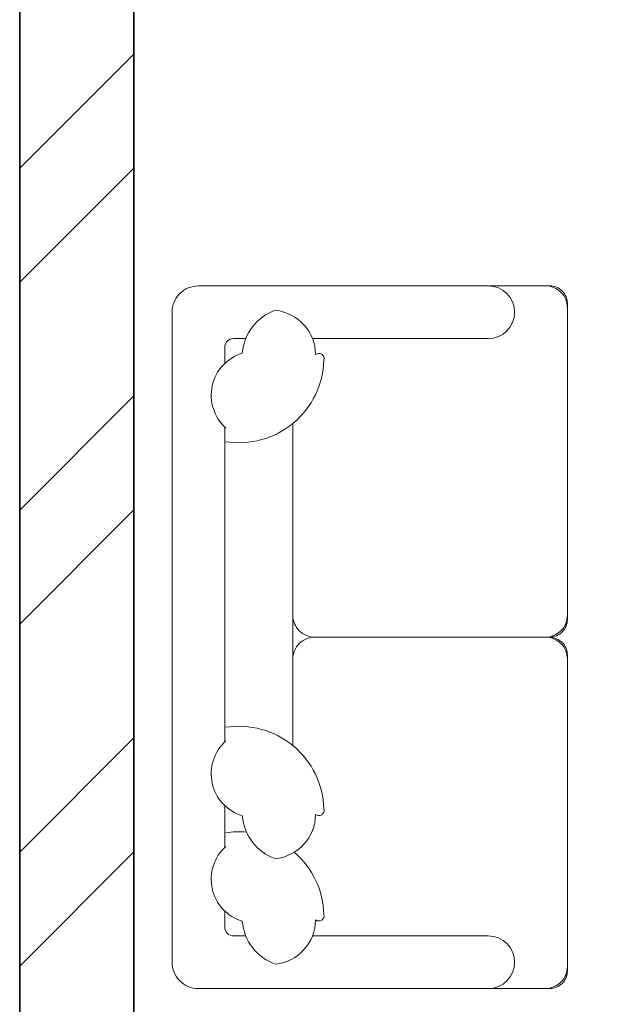
# Model space of a CAD drawing. Units: inches. Extents: x 2168 to 3056, y 1130 to 2629.
# Tile 10 of 42: x 2645 to 2669, y 1979 to 2018. Entities that reach past the tile are written whole.
import ezdxf

# ---------------------------------------------------------------- set-up
doc = ezdxf.new("R2010")
doc.units = ezdxf.units.IN
doc.layers.add('A-FURN', color=8, linetype='Continuous', lineweight=13)
doc.layers.add('A-WALL', color=7, linetype='Continuous', lineweight=35)
doc.layers.add('A-WALL-PATT', color=143, linetype='Continuous', lineweight=13, true_color=0x7aafdf)

msp = doc.modelspace()

# ---------------------------------------------------------------- hatches: boundary and pattern name
at = {"layer": 'A-WALL-PATT'}
h = msp.add_hatch(dxfattribs=at)
h.set_pattern_fill('ANSI32', color=256)
h.paths.add_polyline_path([(2463.796, 2409.389), (2467.387, 2409.389), (2467.387, 2413.889), (2454.768, 2413.889), (2454.768, 2411.639), (2454.768, 2409.389), (2459.296, 2409.389), (2459.296, 2265.389), (2455.644, 2265.389), (2455.644, 2260.889), (2467.349, 2260.889), (2467.349, 2263.139), (2467.349, 2265.389), (2463.796, 2265.389)])
h.paths.add_polyline_path([(2431.596, 2413.889), (2409.647, 2413.889), (2409.647, 2409.389), (2431.596, 2409.389), (2431.596, 2411.639)])
h.paths.add_polyline_path([(2349.647, 2413.889), (2331.796, 2413.889), (2331.796, 2362.671), (2336.296, 2362.671), (2336.296, 2409.389), (2349.647, 2409.389), (2349.647, 2411.639)])
h.paths.add_polyline_path([(2634.149, 2411.639), (2634.149, 2413.889), (2562.293, 2413.889), (2562.293, 2409.389), (2595.796, 2409.389), (2595.796, 2280.309), (2595.826, 2280.309), (2595.826, 2265.389), (2499.91, 2265.389), (2499.91, 2260.889), (2550.796, 2260.889), (2550.796, 2117.308), (2555.296, 2117.308), (2555.296, 2168.08), (2571.93, 2168.08), (2571.93, 2176.889), (2559.796, 2176.889), (2559.796, 2256.389), (2640.796, 2256.389), (2640.796, 2176.889), (2626.428, 2176.889), (2626.428, 2168.08), (2645.296, 2168.08), (2645.296, 2116.637), (2649.796, 2116.637), (2649.796, 2260.889), (2691.251, 2260.889), (2691.251, 2263.139), (2691.251, 2265.389), (2670.655, 2265.389), (2670.655, 2265.365), (2600.296, 2265.365), (2600.296, 2280.258), (2600.296, 2409.389), (2634.149, 2409.389)])
h.paths.add_polyline_path([(2600.296, 2473.889), (2612.84, 2473.889), (2612.84, 2478.389), (2572.636, 2478.389), (2572.636, 2473.889), (2595.796, 2473.889), (2595.796, 2413.889), (2600.296, 2413.889)])
h.paths.add_polyline_path([(2535.796, 2473.889), (2548.636, 2473.889), (2548.636, 2478.389), (2531.396, 2478.389), (2531.396, 2413.889), (2521.6, 2413.889), (2521.6, 2409.389), (2539.239, 2409.389), (2539.239, 2411.639), (2539.239, 2413.889), (2535.796, 2413.889)])
h.paths.add_polyline_path([(2664.796, 2478.389), (2636.84, 2478.389), (2636.84, 2473.889), (2660.296, 2473.889), (2660.296, 2413.889), (2656.165, 2413.889), (2656.165, 2409.389), (2671.684, 2409.389), (2671.684, 2411.639), (2671.684, 2413.889), (2664.796, 2413.889)])
h.paths.add_polyline_path([(2705.942, 2413.889), (2695.684, 2413.889), (2695.684, 2409.389), (2705.942, 2409.389)])
h.paths.add_polyline_path([(2741.35, 2413.889), (2728.733, 2413.889), (2728.733, 2411.639), (2728.733, 2409.389), (2732.296, 2409.389), (2732.296, 2265.389), (2725.733, 2265.389), (2725.733, 2260.889), (2740.917, 2260.889), (2740.917, 2263.139), (2740.917, 2265.389), (2736.796, 2265.389), (2736.796, 2409.389), (2741.35, 2409.389)])
h.paths.add_polyline_path([(2785.655, 2413.889), (2764.546, 2413.889), (2764.486, 2409.389), (2785.655, 2409.389), (2785.655, 2411.639)])
h.paths.add_polyline_path([(2864.296, 2413.889), (2845.655, 2413.889), (2845.655, 2409.389), (2859.796, 2409.389), (2859.796, 2368.425), (2864.296, 2368.425)])
h.paths.add_polyline_path([(2864.296, 2308.425), (2862.046, 2308.425), (2859.796, 2308.425), (2859.796, 2265.389), (2774.483, 2265.389), (2774.483, 2263.139), (2774.483, 2260.889), (2781.796, 2260.889), (2781.796, 2226.654), (2786.296, 2226.654), (2786.296, 2260.889), (2859.796, 2260.889), (2859.796, 2241.352), (2864.296, 2241.352)])
h.paths.add_polyline_path([(2864.296, 2217.352), (2862.046, 2217.352), (2859.796, 2217.352), (2859.796, 2200.889), (2786.296, 2200.889), (2786.296, 2205.931), (2784.046, 2205.931), (2781.796, 2205.931), (2781.796, 2150.974), (2786.296, 2150.974), (2786.296, 2161.889), (2859.796, 2161.889), (2859.796, 2144.419), (2864.296, 2144.419)])
h.paths.add_polyline_path([(2859.796, 2196.389), (2859.796, 2166.389), (2786.296, 2166.389), (2786.296, 2196.389)], flags=16)
h.paths.add_polyline_path([(2864.296, 2108.419), (2862.046, 2108.419), (2859.796, 2108.419), (2859.796, 2080.889), (2786.296, 2080.889), (2786.296, 2111.993), (2781.796, 2111.993), (2781.796, 2080.889), (2649.796, 2080.889), (2649.796, 2086.036), (2647.546, 2086.036), (2645.296, 2086.036), (2645.296, 2071.739), (2649.796, 2071.739), (2649.796, 2076.389), (2781.796, 2076.389), (2781.796, 2041.792), (2786.296, 2041.792), (2786.296, 2076.389), (2859.796, 2076.389), (2859.796, 2058.577), (2864.296, 2058.577)])
h.paths.add_polyline_path([(2864.296, 2022.577), (2859.796, 2022.577), (2859.796, 1992.389), (2786.296, 1992.389), (2786.296, 1999.573), (2781.796, 1999.573), (2781.796, 1848.085), (2784.046, 1848.085), (2786.296, 1848.085), (2786.296, 1851.389), (2859.796, 1851.389), (2859.796, 1838.258), (2864.296, 1838.258)], flags=17)
h.paths.add_polyline_path([(2859.796, 1987.889), (2859.796, 1855.889), (2786.296, 1855.889), (2786.296, 1987.889)], flags=16)
h.paths.add_polyline_path([(2823.046, 1987.889), (2841.421, 1921.889), (2823.046, 1855.889)], flags=0)
h.paths.add_polyline_path([(2864.296, 1814.258), (2859.796, 1814.258), (2859.796, 1791.389), (2786.296, 1791.389), (2786.296, 1825.658), (2784.046, 1825.658), (2781.796, 1825.658), (2781.796, 1791.389), (2720.155, 1791.389), (2720.155, 1791.265), (2649.796, 1791.265), (2649.796, 1806.159), (2649.796, 2038.983), (2647.546, 2038.983), (2645.296, 2038.983), (2645.296, 1783.925), (2649.796, 1783.925), (2649.796, 1786.889), (2781.796, 1786.889), (2781.796, 1746.789), (2786.296, 1746.789), (2786.296, 1786.889), (2859.796, 1786.889), (2859.796, 1770.083), (2864.296, 1770.083)])
h.paths.add_polyline_path([(2864.296, 1734.083), (2862.046, 1734.083), (2859.796, 1734.083), (2859.796, 1705.889), (2786.296, 1705.889), (2786.296, 1714.166), (2781.796, 1714.166), (2781.796, 1660.527), (2786.296, 1660.527), (2786.296, 1666.889), (2859.796, 1666.889), (2859.796, 1648.342), (2864.296, 1648.342)])
h.paths.add_polyline_path([(2786.296, 1701.389), (2859.796, 1701.389), (2859.796, 1671.389), (2786.296, 1671.389)], flags=16)
h.paths.add_polyline_path([(2649.796, 1756.576), (2647.546, 1756.576), (2645.296, 1756.576), (2645.296, 1606.889), (2555.296, 1606.889), (2555.296, 1749.513), (2553.046, 1749.513), (2550.796, 1749.513), (2550.796, 1606.889), (2503.006, 1606.889), (2503.006, 1604.639), (2503.006, 1602.389), (2595.796, 1602.389), (2595.849, 1602.389), (2595.849, 1587.495), (2595.796, 1458.389), (2561.502, 1458.389), (2561.502, 1456.139), (2561.502, 1453.889), (2595.796, 1453.889), (2595.796, 1381.889), (2573.438, 1381.889), (2573.438, 1377.389), (2613.01, 1377.389), (2613.01, 1379.639), (2613.01, 1381.889), (2600.296, 1381.889), (2600.296, 1453.889), (2634.327, 1453.889), (2634.327, 1458.389), (2600.296, 1458.389), (2600.296, 1602.389), (2670.655, 1602.389), (2694.095, 1602.389), (2694.095, 1606.889), (2649.796, 1606.889)])
h.paths.add_polyline_path([(2736.796, 1602.389), (2741.562, 1602.389), (2741.562, 1606.889), (2726.203, 1606.889), (2726.203, 1604.639), (2726.203, 1602.389), (2732.296, 1602.389), (2732.296, 1458.389), (2727.899, 1458.389), (2727.899, 1453.889), (2740.821, 1453.889), (2740.821, 1456.139), (2740.821, 1458.389), (2736.796, 1458.389)])
h.paths.add_polyline_path([(2859.796, 1606.889), (2786.296, 1606.889), (2786.296, 1637.334), (2784.046, 1637.334), (2781.796, 1637.334), (2781.796, 1606.889), (2775.612, 1606.889), (2775.612, 1602.389), (2859.796, 1602.389)])
h.paths.add_polyline_path([(2864.296, 1624.342), (2862.046, 1624.342), (2859.796, 1624.342), (2859.796, 1570.39), (2864.296, 1570.39)])
h.paths.add_polyline_path([(2864.296, 1510.39), (2862.046, 1510.39), (2859.796, 1510.39), (2859.796, 1458.389), (2846.735, 1458.389), (2846.735, 1456.139), (2846.735, 1453.889), (2864.296, 1453.889)])
h.paths.add_polyline_path([(2786.735, 1458.389), (2765.444, 1458.389), (2765.444, 1453.889), (2786.735, 1453.889)])
h.paths.add_polyline_path([(2706.004, 1458.389), (2695.36, 1458.389), (2695.36, 1453.889), (2706.004, 1453.889), (2706.004, 1456.139)])
h.paths.add_polyline_path([(2671.36, 1456.139), (2671.36, 1458.389), (2655.986, 1458.389), (2655.986, 1456.139), (2655.986, 1453.889), (2660.296, 1453.889), (2660.296, 1381.889), (2637.01, 1381.889), (2637.01, 1377.389), (2664.796, 1377.389), (2664.796, 1453.889), (2671.36, 1453.889)], flags=17)
h.paths.add_polyline_path([(2539.829, 1458.389), (2520.237, 1458.389), (2520.237, 1453.889), (2531.296, 1453.889), (2531.296, 1377.389), (2546.449, 1377.389), (2546.449, 1379.639), (2546.449, 1381.889), (2535.796, 1381.889), (2535.796, 1453.889), (2539.829, 1453.889)], flags=17)
h.paths.add_polyline_path([(2496.237, 1458.389), (2489.13, 1458.389), (2489.13, 1453.889), (2496.237, 1453.889), (2496.237, 1456.139)])
h.paths.add_polyline_path([(2467.433, 1456.139), (2467.433, 1458.389), (2463.796, 1458.389), (2463.796, 1602.389), (2468.242, 1602.389), (2468.242, 1605.7), (2468.242, 1606.889), (2454.602, 1606.889), (2454.602, 1602.389), (2459.296, 1602.389), (2459.296, 1458.389), (2454.24, 1458.389), (2454.24, 1453.889), (2467.433, 1453.889)])
h.paths.add_polyline_path([(2431.601, 1456.139), (2431.601, 1458.389), (2411.386, 1458.389), (2411.386, 1453.889), (2431.601, 1453.889)])
h.paths.add_polyline_path([(2351.386, 1458.389), (2336.296, 1458.389), (2336.296, 1490.693), (2334.046, 1490.693), (2331.796, 1490.693), (2331.796, 1453.889), (2351.386, 1453.889), (2351.386, 1456.139)])
h.paths.add_polyline_path([(2336.296, 1629.705), (2331.796, 1629.705), (2331.796, 1552.317), (2336.296, 1552.317), (2336.296, 1602.389), (2406.655, 1602.389), (2423.472, 1602.389), (2423.472, 1606.889), (2418.796, 1606.889), (2418.796, 1643.678), (2416.546, 1643.678), (2414.296, 1643.678), (2414.296, 1606.889), (2336.296, 1606.889)])
h.paths.add_polyline_path([(2418.796, 1714.384), (2414.296, 1714.384), (2414.296, 1705.889), (2336.296, 1705.889), (2336.296, 1731.324), (2334.046, 1731.324), (2331.796, 1731.324), (2331.796, 1653.705), (2334.046, 1653.705), (2336.296, 1653.705), (2336.296, 1666.889), (2414.296, 1666.889), (2414.296, 1663.589), (2418.796, 1663.589)])
h.paths.add_polyline_path([(2336.296, 1701.389), (2414.296, 1701.389), (2414.296, 1671.389), (2336.296, 1671.389)], flags=16)
h.paths.add_polyline_path([(2555.296, 2040.059), (2550.796, 2040.059), (2550.796, 1791.389), (2550.561, 1791.205), (2480.202, 1791.205), (2418.796, 1791.389), (2418.796, 1825.448), (2416.546, 1825.448), (2414.296, 1825.448), (2414.296, 1791.389), (2336.296, 1791.389), (2336.296, 1806.409), (2331.796, 1806.409), (2331.796, 1767.324), (2336.296, 1767.324), (2336.296, 1786.889), (2414.296, 1786.889), (2414.296, 1745.457), (2418.796, 1745.457), (2418.796, 1786.889), (2550.796, 1786.889), (2550.796, 1783.011), (2555.296, 1783.011)])
h.paths.add_polyline_path([(2418.796, 1923.389), (2423.207, 1923.389), (2423.207, 1925.639), (2423.207, 1927.889), (2418.796, 1927.889), (2418.796, 2000.048), (2414.296, 2000.048), (2414.296, 1992.389), (2336.296, 1992.389), (2336.296, 1987.889), (2414.296, 1987.889), (2414.296, 1855.889), (2336.296, 1855.889), (2336.296, 1851.389), (2414.296, 1851.389), (2414.296, 1846.759), (2418.796, 1846.759)], flags=17)
h.paths.add_polyline_path([(2336.296, 2019.294), (2334.046, 2019.294), (2331.796, 2019.294), (2331.796, 1830.409), (2336.296, 1830.409)], flags=17)
h.paths.add_polyline_path([(2550.796, 1927.889), (2453.541, 1927.889), (2453.541, 1925.639), (2453.541, 1923.389), (2550.796, 1923.389)], flags=17)
h.paths.add_polyline_path([(2744.987, 1927.889), (2649.796, 1927.889), (2649.796, 1923.389), (2744.987, 1923.389), (2744.987, 1925.639)], flags=17)
h.paths.add_polyline_path([(2555.296, 2086.458), (2553.046, 2086.458), (2550.796, 2086.458), (2550.796, 2080.889), (2418.796, 2080.889), (2336.296, 2080.889), (2336.296, 2115.399), (2334.046, 2115.399), (2331.796, 2115.399), (2331.796, 2055.294), (2336.296, 2055.294), (2336.296, 2076.389), (2550.796, 2076.389), (2550.796, 2071.538), (2555.296, 2071.538)])
h.paths.add_polyline_path([(2418.796, 2121.389), (2414.296, 2121.389), (2414.296, 2080.889), (2418.796, 2080.889)])
h.paths.add_polyline_path([(2418.796, 2076.389), (2414.296, 2076.389), (2414.296, 2035.123), (2418.796, 2035.123)])
h.paths.add_polyline_path([(2422.868, 2263.139), (2422.868, 2265.389), (2406.655, 2265.389), (2406.655, 2265.359), (2336.296, 2265.359), (2336.296, 2280.252), (2336.296, 2302.671), (2334.046, 2302.671), (2331.796, 2302.671), (2331.796, 2246.853), (2336.296, 2246.853), (2336.296, 2260.889), (2414.296, 2260.889), (2414.296, 2223.996), (2418.796, 2223.996), (2418.796, 2260.889), (2422.868, 2260.889)])
h.paths.add_polyline_path([(2418.796, 2204.783), (2416.546, 2204.783), (2414.296, 2204.783), (2414.296, 2200.889), (2336.296, 2200.889), (2336.296, 2220.853), (2331.796, 2220.853), (2331.796, 2151.399), (2336.296, 2151.399), (2336.296, 2161.889), (2414.296, 2161.889), (2414.296, 2153.726), (2418.796, 2153.726)])
h.paths.add_polyline_path([(2414.296, 2196.389), (2414.296, 2166.389), (2336.296, 2166.389), (2336.296, 2196.389)], flags=16)
h.paths.add_polyline_path([(2375.296, 2181.389), (2336.296, 2166.389), (2336.296, 2196.389)], flags=0)
h.paths.add_polyline_path([(2809.595, 2172.34), (2838.804, 2172.34), (2838.804, 2190.997), (2809.595, 2190.997)], flags=8)
h.paths.add_polyline_path([(2849.75, 1919.585), (2849.75, 1952.672), (2831.093, 1952.672), (2831.093, 1919.585)], flags=8)
h.paths.add_polyline_path([(2808.875, 1901.967), (2808.875, 1937.85), (2790.149, 1937.85), (2790.149, 1901.967)], flags=8)
h.paths.add_polyline_path([(2806.285, 1671.896), (2835.493, 1671.896), (2835.493, 1690.553), (2806.285, 1690.553)], flags=8)
h.paths.add_polyline_path([(2353.186, 1676.549), (2382.395, 1676.549), (2382.395, 1695.207), (2353.186, 1695.207)], flags=8)
h.paths.add_polyline_path([(2360.083, 1832.308), (2389.241, 1832.308), (2389.241, 1850.966), (2360.083, 1850.966)], flags=25)
h.paths.add_polyline_path([(2354.822, 2167.823), (2384.031, 2167.823), (2384.031, 2186.481), (2354.822, 2186.481)], flags=8)

# ---------------------------------------------------------------- linework, layer by layer
at = {"layer": 'A-FURN'}
for p, q in [((2653.372, 2005.132), (2653.372, 2004.496)), ((2654.2, 2005.478), (2653.718, 2005.478)), ((2663.754, 2005.478), (2656.826, 2005.478)), ((2653.372, 2001.998), (2653.372, 1989.582)), ((2653.372, 1986.447), (2653.372, 1987.084)), ((2653.372, 1987.084), (2653.372, 1985.428)), ((2653.372, 1982.293), (2653.372, 1982.93)), ((2654.2, 1981.947), (2653.718, 1981.947)), ((2656.826, 1981.947), (2663.754, 1981.947))]:
    msp.add_line(p, q, dxfattribs=at)
at = {"layer": 'A-FURN', "ltscale": 0.03}
msp.add_lwpolyline([(2666.176, 1993.721, 0.414214), (2666.868, 1994.413), (2666.868, 2006.863, 0.414214), (2666.176, 2007.555), (2652.334, 2007.555, 0.414214), (2651.296, 2006.517), (2651.296, 1980.909, 0.414214), (2652.334, 1979.871), (2666.176, 1979.871, 0.414214), (2666.868, 1980.563), (2666.868, 1993.012, 0.414214), (2666.176, 1993.704)], format="xyb", dxfattribs=at)
at = {"layer": 'A-FURN'}
for points in [[(2656.054, 2001.547), (2656.054, 1994.578, 0.414214), (2656.919, 1993.713), (2666.003, 1993.713, 0.414214), (2666.868, 1994.578), (2666.868, 2006.69, 0.414214), (2666.003, 2007.555)], [(2656.054, 1989.443), (2656.054, 1992.848, -0.414214), (2656.919, 1993.713), (2666.003, 1993.713, -0.414214), (2666.868, 1992.848), (2666.868, 1980.736, -0.414214), (2666.003, 1979.871)]]:
    msp.add_lwpolyline(points, format="xyb", dxfattribs=at)
msp.add_lwpolyline([(2656.054, 1989.443), (2656.054, 2002.136)], dxfattribs=at)
for centre, radius, start, end in [((2663.754, 2006.517), 1.038, 0, 90), ((2656.01, 2004.749), 1.951, 109.1026, 175.4561), ((2655.172, 2004.826), 1.778, 0.743, 83.5721), ((2663.754, 2006.517), 1.038, 270, 0), ((2653.718, 2005.132), 0.346, 90, 180), ((2654.574, 2003.247), 1.734, 107.0949, 228.2428), ((2657.077, 2004.686), 0.207, 344.7265, 127.845), ((2653.929, 2004.726), 3.35, 261.117, 358.3884), ((2653.929, 1986.854), 3.35, 1.6116, 98.883), ((2654.574, 1988.333), 1.734, 131.7572, 252.9051), ((2657.077, 1986.894), 0.207, 232.155, 15.2735), ((2656.01, 1986.831), 1.951, 184.5439, 250.8974), ((2655.172, 1986.753), 1.778, 276.4279, 359.257), ((2653.929, 1982.7), 3.35, 84.881, 98.883), ((2654.574, 1984.179), 1.734, 131.7572, 252.9051), ((2653.929, 1982.7), 3.35, 1.6116, 49.376), ((2657.077, 1982.74), 0.207, 232.155, 15.2735), ((2653.718, 1982.293), 0.346, 180, 270), ((2653.718, 1982.293), 0.346, 180, 270), ((2656.01, 1982.676), 1.951, 184.5439, 250.8974), ((2655.172, 1982.599), 1.778, 276.4279, 359.257), ((2663.754, 1980.909), 1.038, 0, 90), ((2663.754, 1980.909), 1.038, 270, 0)]:
    msp.add_arc(centre, radius, start, end, dxfattribs=at)
at = {"layer": 'A-WALL'}
for p, q in [((2649.796, 1791.389), (2649.796, 2040.564)), ((2645.296, 2038.983), (2645.296, 1783.925))]:
    msp.add_line(p, q, dxfattribs=at)

doc.saveas('drawing.dxf')
